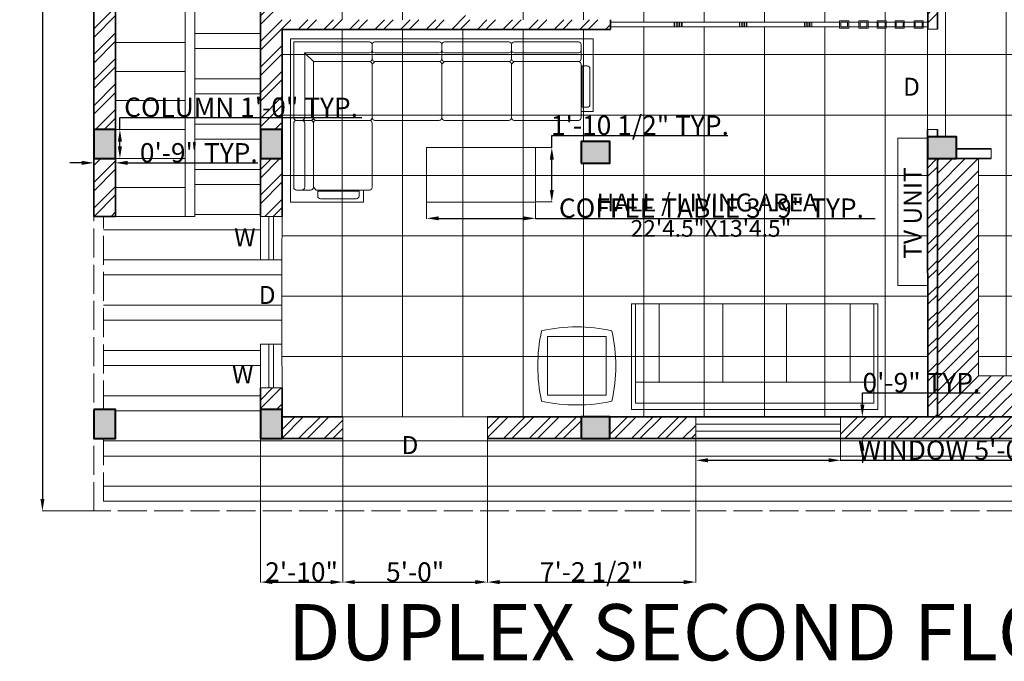
# Model space of a CAD drawing. Units: inches. Extents: x 351 to 1738, y -265 to 286.
# Tile 1 of 38: x 351 to 759, y -265 to 0. Entities that reach past the tile are written whole.
import ezdxf

# ---------------------------------------------------------------- set-up
doc = ezdxf.new("R2010")
doc.units = ezdxf.units.IN
doc.header["$MEASUREMENT"] = 0
doc.linetypes.add('ACAD_ISO02W100', pattern=[15, 12, -3])
doc.linetypes.add('ACAD_ISO03W100', pattern=[30, 12, -18])
for name, color, linetype, lineweight in [('A-ANNO-DIMS', 2, 'Continuous', 18), ('A-ANNO-SYMB', 7, 'Continuous', 18), ('A-ANNO-TEXT', 7, 'Continuous', 18), ('A-ANNO-TITL', 7, 'Continuous', 35), ('A-AREA-IDEN', 7, 'Continuous', 18), ('A-COLS', 7, 'Continuous', 40), ('A-COLS-PATT', 6, 'Continuous', 13), ('A-DOOR', 3, 'Continuous', 18), ('A-DOOR-HIDN', 3, 'ACAD_ISO03W100', 13), ('A-DOOR-OVHD', 3, 'ACAD_ISO02W100', 13), ('A-FLOR-CASE', 9, 'Continuous', 18), ('A-FLOR-CASE-PATT', 9, 'Continuous', 9), ('A-FLOR-OVHD', 1, 'ACAD_ISO02W100', 18), ('A-FLOR-PATT', 9, 'Continuous', 9), ('A-FLOR-STRS', 7, 'Continuous', 18), ('A-FURN', 18, 'Continuous', 13), ('A-GLAZ', 4, 'Continuous', 18), ('A-WALL', 7, 'Continuous', 35), ('A-WALL-PATT', 152, 'Continuous', 13), ('A-WALL-SCRN', 7, 'Continuous', 18), ('A-WALL-SCRN-PATT', 30, 'Continuous', 13)]:
    doc.layers.add(name, color=color, linetype=linetype, lineweight=lineweight)
doc.styles.add('Annotative', font='arial.ttf')
doc.styles.get("Standard").update_dxf_attribs({"font": 'arial.ttf'})
doc.dimstyles.get("Standard").update_dxf_attribs({"dimtxt": 8, "dimasz": 5, "dimexe": 0.18, "dimexo": 0.0625, "dimgap": 0.09, "dimtad": 1, "dimtoh": 1, "dimzin": 0, "dimdsep": 46, "dimlunit": 4, "dimtxsty": 'Standard', "dimcen": 0, "dimclre": 256, "dimadec": 0, "dimazin": 0, "dimtfac": 1, "dimtofl": 0, "dimtmove": 0, "dimatfit": 3, "dimfxl": 1, "dimtolj": 1, "dimtzin": 0, "dimlwe": -1, "dimarcsym": 0})

# ---------------------------------------------------------------- blocks, each defined once
blk = doc.blocks.new('*D3')
at = {"layer": 'A-ANNO-DIMS', "color": 0, "transparency": 16777216}
for p, q in [((382.09, 255.96), (360.67, 255.96)), ((382.09, -203.04), (360.67, -203.04))]:
    blk.add_line(p, q, dxfattribs=at)
at = {"layer": 'A-ANNO-DIMS', "color": 0, "lineweight": -2, "transparency": 16777216}
blk.add_line((360.85, 250.96), (360.85, -198.04), dxfattribs=at)
at = {"layer": 'A-ANNO-DIMS', "color": 0, "transparency": 16777216}
for points in [[(360.02, 250.96), (361.69, 250.96), (360.85, 255.96)], [(360.02, -198.04), (361.69, -198.04), (360.85, -203.04)]]:
    blk.add_solid(points, dxfattribs=at)
at = {"layer": 'Defpoints', "color": 0, "transparency": 16777216}
for p in [(382.16, 255.96), (360.85, -203.04), (382.16, -203.04)]:
    blk.add_point(p, dxfattribs=at)
at = {"layer": 'A-ANNO-DIMS', "color": 0, "transparency": 16777216, "insert": (356.68, 26.46), "char_height": 8, "attachment_point": 5, "rotation": 90}
blk.add_mtext('\\A1;38\'-3"', dxfattribs=at)
blk = doc.blocks.new('TABLE-COFFEE-RECT')
blk.add_lwpolyline([(0, 0), (0, 22.55), (45.11, 22.55), (45.11, 0)], close=True)
blk = doc.blocks.new('CONSOLE-TV')
blk.add_lwpolyline([(0, 0), (61, 0), (61, 12.29), (0, 12.29)], close=True)
blk = doc.blocks.new('COL-9x12')
blk.add_lwpolyline([(0, 12), (0, 0), (9, 0), (9, 12)], close=True)
blk = doc.blocks.new('WIN-60')
for p, q in [((0, 6), (60, 6)), ((0, 3), (60, 3))]:
    blk.add_line(p, q)
blk.add_lwpolyline([(60, 0), (60, 9), (0, 9), (0, 0)], close=True)
blk = doc.blocks.new('*D30')
at = {"layer": 'A-ANNO-DIMS', "color": 0, "lineweight": -2, "transparency": 16777216}
for p, q in [((392.96, -45.04), (392.96, -40.04)), ((392.96, -40.04), (493.25, -40.04)), ((392.96, -52.04), (392.96, -50.04))]:
    blk.add_line(p, q, dxfattribs=at)
at = {"layer": 'A-ANNO-DIMS', "transparency": 16777216}
for p, q in [((391.22, -45.04), (393.14, -45.04)), ((391.22, -57.04), (393.14, -57.04))]:
    blk.add_line(p, q, dxfattribs=at)
at = {"layer": 'A-ANNO-DIMS', "color": 0, "transparency": 16777216}
for points in [[(392.12, -50.04), (393.79, -50.04), (392.96, -45.04)], [(392.12, -52.04), (393.79, -52.04), (392.96, -57.04)]]:
    blk.add_solid(points, dxfattribs=at)
at = {"layer": 'Defpoints', "color": 0, "transparency": 16777216}
for p in [(391.16, -45.04), (392.96, -45.04), (391.16, -57.04)]:
    blk.add_point(p, dxfattribs=at)
at = {"layer": 'A-ANNO-DIMS', "color": 0, "transparency": 16777216, "insert": (443.15, -35.81), "char_height": 8, "attachment_point": 5}
blk.add_mtext('\\A1;COLUMN 1\'-0" TYP.', dxfattribs=at)
blk = doc.blocks.new('*D31')
at = {"layer": 'A-ANNO-DIMS', "transparency": 16777216}
for p, q in [((382.16, -57.1), (382.16, -59.02)), ((391.16, -57.1), (391.16, -59.02))]:
    blk.add_line(p, q, dxfattribs=at)
at = {"layer": 'A-ANNO-DIMS', "color": 0, "lineweight": -2, "transparency": 16777216}
for p, q in [((377.16, -58.84), (372.16, -58.84)), ((396.16, -58.84), (450.1, -58.84))]:
    blk.add_line(p, q, dxfattribs=at)
at = {"layer": 'A-ANNO-DIMS', "color": 0, "transparency": 16777216}
for points in [[(377.16, -58), (377.16, -59.67), (382.16, -58.84)], [(396.16, -58), (396.16, -59.67), (391.16, -58.84)]]:
    blk.add_solid(points, dxfattribs=at)
at = {"layer": 'Defpoints', "color": 0, "transparency": 16777216}
for p in [(382.16, -57.04), (391.16, -57.04), (391.16, -58.84)]:
    blk.add_point(p, dxfattribs=at)
at = {"layer": 'A-ANNO-DIMS', "color": 0, "transparency": 16777216, "insert": (425.63, -54.66), "char_height": 8, "attachment_point": 5}
blk.add_mtext('\\A1;0\'-9" TYP.', dxfattribs=at)
blk = doc.blocks.new('*D34')
at = {"layer": 'A-ANNO-DIMS', "transparency": 16777216}
for p, q in [((631.58, -173.1), (631.58, -182.22)), ((691.58, -173.1), (691.58, -182.22))]:
    blk.add_line(p, q, dxfattribs=at)
at = {"layer": 'A-ANNO-DIMS', "color": 0, "lineweight": -2, "transparency": 16777216}
for p, q in [((636.58, -182.04), (686.58, -182.04)), ((691.58, -182.04), (797.99, -182.04))]:
    blk.add_line(p, q, dxfattribs=at)
at = {"layer": 'A-ANNO-DIMS', "color": 0, "transparency": 16777216}
for points in [[(636.58, -181.2), (636.58, -182.87), (631.58, -182.04)], [(686.58, -181.2), (686.58, -182.87), (691.58, -182.04)]]:
    blk.add_solid(points, dxfattribs=at)
at = {"layer": 'Defpoints', "color": 0, "transparency": 16777216}
for p in [(631.58, -173.04), (691.58, -173.04), (691.58, -182.04)]:
    blk.add_point(p, dxfattribs=at)
at = {"layer": 'A-ANNO-DIMS', "color": 0, "transparency": 16777216, "insert": (747.29, -177.81), "char_height": 8, "attachment_point": 5}
blk.add_mtext('\\A1;WINDOW 5\'-0" TYP.', dxfattribs=at)
blk = doc.blocks.new('*D35')
at = {"layer": 'A-ANNO-DIMS', "color": 0, "lineweight": -2, "transparency": 16777216}
for p, q in [((700.58, -159.04), (700.58, -154.04)), ((700.58, -154.04), (749.43, -154.04)), ((700.58, -178.04), (700.58, -183.04))]:
    blk.add_line(p, q, dxfattribs=at)
at = {"layer": 'A-ANNO-DIMS', "transparency": 16777216}
for p, q in [((691.64, -164.04), (700.76, -164.04)), ((691.64, -173.04), (700.76, -173.04))]:
    blk.add_line(p, q, dxfattribs=at)
at = {"layer": 'A-ANNO-DIMS', "color": 0, "transparency": 16777216}
for points in [[(699.75, -159.04), (701.41, -159.04), (700.58, -164.04)], [(699.75, -178.04), (701.41, -178.04), (700.58, -173.04)]]:
    blk.add_solid(points, dxfattribs=at)
at = {"layer": 'Defpoints', "color": 0, "transparency": 16777216}
for p in [(691.58, -164.04), (700.58, -164.04), (691.58, -173.04)]:
    blk.add_point(p, dxfattribs=at)
at = {"layer": 'A-ANNO-DIMS', "color": 0, "transparency": 16777216, "insert": (725.05, -149.86), "char_height": 8, "attachment_point": 5}
blk.add_mtext('\\A1;0\'-9" TYP.', dxfattribs=at)
blk = doc.blocks.new('*D50')
at = {"layer": 'A-ANNO-DIMS', "transparency": 16777216}
for p, q in [((520.02, -75.12), (520.02, -82)), ((565.13, -75.12), (565.13, -82))]:
    blk.add_line(p, q, dxfattribs=at)
at = {"layer": 'A-ANNO-DIMS', "color": 0, "lineweight": -2, "transparency": 16777216}
for p, q in [((525.02, -81.82), (560.13, -81.82)), ((565.13, -81.82), (705.92, -81.82))]:
    blk.add_line(p, q, dxfattribs=at)
at = {"layer": 'A-ANNO-DIMS', "color": 0, "transparency": 16777216}
for points in [[(525.02, -80.99), (525.02, -82.65), (520.02, -81.82)], [(560.13, -80.99), (560.13, -82.65), (565.13, -81.82)]]:
    blk.add_solid(points, dxfattribs=at)
at = {"layer": 'Defpoints', "color": 0, "transparency": 16777216}
for p in [(520.02, -75.05), (565.13, -75.05), (565.13, -81.82)]:
    blk.add_point(p, dxfattribs=at)
at = {"layer": 'A-ANNO-DIMS', "color": 0, "transparency": 16777216, "insert": (638.03, -77.59), "char_height": 8, "attachment_point": 5}
blk.add_mtext('\\A1;COFFEE TABLE 3\'-9" TYP.', dxfattribs=at)
blk = doc.blocks.new('*D51')
at = {"layer": 'A-ANNO-DIMS', "color": 0, "lineweight": -2, "transparency": 16777216}
for p, q in [((571.9, -52.5), (571.9, -47.5)), ((571.9, -47.5), (644.85, -47.5)), ((571.9, -70.05), (571.9, -57.5))]:
    blk.add_line(p, q, dxfattribs=at)
at = {"layer": 'A-ANNO-DIMS', "transparency": 16777216}
for p, q in [((565.19, -52.5), (572.08, -52.5)), ((565.19, -75.05), (572.08, -75.05))]:
    blk.add_line(p, q, dxfattribs=at)
at = {"layer": 'A-ANNO-DIMS', "color": 0, "transparency": 16777216}
for points in [[(571.06, -57.5), (572.73, -57.5), (571.9, -52.5)], [(571.06, -70.05), (572.73, -70.05), (571.9, -75.05)]]:
    blk.add_solid(points, dxfattribs=at)
at = {"layer": 'Defpoints', "color": 0, "transparency": 16777216}
for p in [(565.13, -52.5), (571.9, -52.5), (565.13, -75.05)]:
    blk.add_point(p, dxfattribs=at)
at = {"layer": 'A-ANNO-DIMS', "color": 0, "transparency": 16777216, "insert": (608.42, -43.28), "char_height": 8, "attachment_point": 5}
blk.add_mtext('\\A1;1\'-10 1/2" TYP.', dxfattribs=at)
blk = doc.blocks.new('*D56')
at = {"layer": 'A-ANNO-DIMS', "transparency": 16777216}
for p, q in [((451.16, -173.1), (451.16, -232.67)), ((485.28, -173.1), (485.28, -232.67))]:
    blk.add_line(p, q, dxfattribs=at)
at = {"layer": 'A-ANNO-DIMS', "color": 0, "lineweight": -2, "transparency": 16777216}
blk.add_line((456.16, -232.49), (480.28, -232.49), dxfattribs=at)
at = {"layer": 'A-ANNO-DIMS', "color": 0, "transparency": 16777216}
for points in [[(456.16, -231.65), (456.16, -233.32), (451.16, -232.49)], [(480.28, -231.65), (480.28, -233.32), (485.28, -232.49)]]:
    blk.add_solid(points, dxfattribs=at)
at = {"layer": 'Defpoints', "color": 0, "transparency": 16777216}
for p in [(451.16, -173.04), (485.28, -173.04), (485.28, -232.49)]:
    blk.add_point(p, dxfattribs=at)
at = {"layer": 'A-ANNO-DIMS', "color": 0, "transparency": 16777216, "insert": (468.22, -228.31), "char_height": 8, "attachment_point": 5}
blk.add_mtext('\\A1;2\'-10"', dxfattribs=at)
blk = doc.blocks.new('*D57')
at = {"layer": 'A-ANNO-DIMS', "transparency": 16777216}
for p, q in [((485.28, -173.1), (485.28, -232.67)), ((545.28, -173.1), (545.28, -232.67))]:
    blk.add_line(p, q, dxfattribs=at)
at = {"layer": 'A-ANNO-DIMS', "color": 0, "lineweight": -2, "transparency": 16777216}
blk.add_line((490.28, -232.49), (540.28, -232.49), dxfattribs=at)
at = {"layer": 'A-ANNO-DIMS', "color": 0, "transparency": 16777216}
for points in [[(490.28, -231.65), (490.28, -233.32), (485.28, -232.49)], [(540.28, -231.65), (540.28, -233.32), (545.28, -232.49)]]:
    blk.add_solid(points, dxfattribs=at)
at = {"layer": 'Defpoints', "color": 0, "transparency": 16777216}
for p in [(485.28, -173.04), (545.28, -173.04), (545.28, -232.49)]:
    blk.add_point(p, dxfattribs=at)
at = {"layer": 'A-ANNO-DIMS', "color": 0, "transparency": 16777216, "insert": (515.28, -228.31), "char_height": 8, "attachment_point": 5}
blk.add_mtext('\\A1;5\'-0"', dxfattribs=at)
blk = doc.blocks.new('*D58')
at = {"layer": 'A-ANNO-DIMS', "transparency": 16777216}
for p, q in [((545.28, -173.1), (545.28, -232.67)), ((631.58, -173.1), (631.58, -232.67))]:
    blk.add_line(p, q, dxfattribs=at)
at = {"layer": 'A-ANNO-DIMS', "color": 0, "lineweight": -2, "transparency": 16777216}
blk.add_line((550.28, -232.49), (626.58, -232.49), dxfattribs=at)
at = {"layer": 'A-ANNO-DIMS', "color": 0, "transparency": 16777216}
for points in [[(550.28, -231.65), (550.28, -233.32), (545.28, -232.49)], [(626.58, -231.65), (626.58, -233.32), (631.58, -232.49)]]:
    blk.add_solid(points, dxfattribs=at)
at = {"layer": 'Defpoints', "color": 0, "transparency": 16777216}
for p in [(545.28, -173.04), (631.58, -173.04), (631.58, -232.49)]:
    blk.add_point(p, dxfattribs=at)
at = {"layer": 'A-ANNO-DIMS', "color": 0, "transparency": 16777216, "insert": (588.43, -228.26), "char_height": 8, "attachment_point": 5}
blk.add_mtext('\\A1;7\'-2 1/2"', dxfattribs=at)

msp = doc.modelspace()

# ---------------------------------------------------------------- hatches: boundary and pattern name
at = {"layer": 'A-COLS-PATT'}
h = msp.add_hatch(color=256, dxfattribs=at)
h.dxf.hatch_style = 1
h.paths.add_polyline_path([(460.155, 237.963), (451.155, 237.963), (451.155, 228.963), (460.155, 228.963)])
h.paths.add_polyline_path([(463.155, 237.963), (460.155, 237.963), (460.155, 228.963), (463.155, 228.963)])
h.paths.add_polyline_path([(391.155, 255.963), (382.155, 255.963), (382.155, 243.963), (391.155, 243.963)])
h.paths.add_polyline_path([(391.155, 210.963), (382.155, 210.963), (382.155, 198.963), (391.155, 198.963)])
h.paths.add_polyline_path([(391.155, -45.037), (382.155, -45.037), (382.155, -57.037), (391.155, -57.037)])
h.paths.add_polyline_path([(460.155, -45.037), (451.155, -45.037), (451.155, -57.037), (460.155, -57.037)])
h.paths.add_polyline_path([(460.155, -161.037), (451.155, -161.037), (451.155, -164.037), (451.155, -173.037), (460.155, -173.037)])
h.paths.add_polyline_path([(391.155, -161.037), (382.155, -161.037), (382.155, -173.037), (391.155, -173.037)])
h.paths.add_polyline_path([(596, -164.037), (584, -164.037), (584, -173.037), (596, -173.037)])
h.paths.add_polyline_path([(596, -50), (584, -50), (584, -59), (596, -59)])
h.paths.add_polyline_path([(596.155, 73.463), (592.155, 73.463), (592.155, 64.463), (596.155, 64.463)])
h.paths.add_polyline_path([(592.155, 73.463), (584.155, 73.463), (584.155, 64.463), (592.155, 64.463)])
h.paths.add_polyline_path([(596.155, 237.963), (584.155, 237.963), (584.155, 228.963), (596.155, 228.963)])
h.paths.add_polyline_path([(739.655, 237.963), (727.655, 237.963), (727.655, 228.963), (739.655, 228.963)])
h.paths.add_polyline_path([(883.515, 237.963), (871.515, 237.963), (871.515, 228.963), (883.515, 228.963)])
h.paths.add_polyline_path([(883.515, 73.463), (871.515, 73.463), (871.515, 64.463), (883.515, 64.463)])
h.paths.add_polyline_path([(731.655, 73.463), (727.655, 73.463), (727.655, 64.463), (731.655, 64.463)])
h.paths.add_polyline_path([(739.515, 73.463), (731.655, 73.463), (731.655, 64.463), (739.515, 64.463)])
h.paths.add_polyline_path([(883.515, -53.037), (871.515, -53.037), (871.515, -57.037), (883.515, -57.037)])
h.paths.add_polyline_path([(883.515, -48.037), (871.515, -48.037), (871.515, -53.037), (883.515, -53.037)])
h.paths.add_polyline_path([(739.515, -48.037), (727.515, -48.037), (727.515, -56.5), (727.516, -57.037), (739.515, -57.037)])
h.paths.add_polyline_path([(883.515, -164.037), (871.515, -164.037), (871.515, -173.037), (883.515, -173.037)])
at = {"layer": 'A-FLOR-CASE-PATT'}
h = msp.add_hatch(dxfattribs=at)
h.set_pattern_fill('ANSI31', color=256, scale=30)
h.set_pattern_definition([(45, (731.6553, -164.0373), (-2.65165, 2.65165), [])])
h.paths.add_polyline_path([(748.655, -57.037), (731.655, -57.037), (731.655, -164.037), (815.655, -164.037), (815.655, -147.037), (748.655, -147.037)])
at = {"layer": 'A-FLOR-PATT', "transparency": 33554559}
h = msp.add_hatch(dxfattribs=at)
h.set_pattern_fill('ANSI37', color=256, scale=200, angle=45)
h.set_pattern_definition([(90, (460.077, -164.037), (-25, 0), []), (180, (460.077, -164.037), (-4e-15, -25), [])])
h.paths.add_polyline_path([(727.516, -57.037), (727.515, -57.037), (727.515, -56.5), (727.5, -45), (727.5, -3.5), (727.501, -2.537), (725.797, -2.537), (725.797, -3.037), (721.988, -3.037), (721.988, -2.537), (717.916, -2.537), (717.916, -3.037), (714.106, -3.037), (714.106, -2.537), (710.487, -2.537), (710.487, -3.037), (706.677, -3.037), (706.677, -2.537), (702.965, -2.537), (702.965, -3.037), (699.155, -3.037), (699.155, -2.537), (694.965, -2.537), (694.965, -3.037), (691.155, -3.037), (691.155, -2.537), (679.655, -2.537), (678.797, -2.537), (677.776, -2.537), (676.723, -2.537), (652.655, -2.537), (651.799, -2.537), (650.778, -2.537), (649.725, -2.537), (625.877, -2.537), (624.879, -2.537), (623.857, -2.537), (622.804, -2.537), (596.155, -2.537), (596.155, -3.537), (460.155, -3.537), (460.155, -81.037), (460.077, -99.07), (460.077, -133.967), (460.155, -152.037), (460.155, -164.037), (485.277, -164.037), (545.277, -164.037), (727.655, -164.037)])
h.paths.add_polyline_path([(584, -59), (584, -50), (596, -50), (596, -59)], flags=16)
h.paths.add_polyline_path([(905.155, 204.963), (731.655, 204.963), (731.655, 73.463), (739.515, 73.463), (739.515, 64.463), (731.655, 64.463), (731.655, -3.5), (727.655, -3.5), (727.655, -3.537), (727.5, -45), (731.655, -45), (731.655, -48.037), (739.515, -48.037), (739.515, -53.037), (754, -53.037), (754, -57.037), (748.655, -57.037), (748.655, -147.037), (815.655, -147.037), (815.655, -138.5), (819.655, -138.5), (819.655, -102.5), (815.655, -102.5), (815.655, -57.037), (790, -57.037), (790, -53.037), (871.515, -53.037), (871.515, -48.037), (883.515, -48.037), (883.515, -53.037), (905.155, -53.037)])
h.paths.add_polyline_path([(871.515, 64.463), (871.515, 73.463), (883.515, 73.463), (883.515, 64.463)], flags=16)
h.paths.add_polyline_path([(727.655, 64.463), (685.515, 64.463), (685.515, 186.963), (638.155, 186.963), (638.155, 88.463), (596.155, 88.463), (596.155, 64.463), (584.155, 64.463), (584.155, 73.463), (592.155, 73.463), (592.155, 205.963), (574, 205.963), (574, 209.963), (538, 209.963), (538, 205.963), (536.5, 205.963), (536.5, 180), (489.5, 180), (489.5, 68.655), (460.155, 68.655), (460.155, 64.463), (536.155, 64.463), (536.155, 48.463), (532.155, 48.463), (532.155, 60.463), (460.155, 60.463), (460.155, 0.463), (532.155, 0.463), (532.155, 12.463), (536.155, 12.463), (536.155, 0.463), (596.155, 0.463), (596.155, -0.537), (622.655, -0.537), (623.655, -0.537), (624.655, -0.537), (625.655, -0.537), (649.655, -0.537), (650.576, -0.537), (651.576, -0.537), (652.576, -0.537), (676.655, -0.537), (677.574, -0.537), (678.574, -0.537), (679.574, -0.537), (691.155, -0.537), (691.155, -0.037), (694.965, -0.037), (694.965, -0.537), (699.155, -0.537), (699.155, -0.037), (702.965, -0.037), (702.965, -0.537), (706.677, -0.537), (706.677, -0.037), (710.487, -0.037), (710.487, -0.537), (714.106, -0.537), (714.106, -0.037), (717.916, -0.037), (717.916, -0.537), (721.988, -0.537), (721.988, -0.037), (725.797, -0.037), (725.797, -0.537), (727.655, -0.537)])
h.paths.add_polyline_path([(485.401, 6.538), (461.783, 6.538), (461.783, 51.327), (485.401, 51.327)], flags=16)
h.paths.add_polyline_path([(483.401, 8.538), (463.783, 8.538), (463.783, 49.327), (483.401, 49.327)], flags=0)
h.paths.add_polyline_path([(476.907, 30.5), (476.907, 29.5), (476.907, 26), (475.907, 26), (475.907, 29.5), (474.449, 29.5), (474.449, 26), (473.449, 26), (470.5, 26), (470.5, 27), (473.449, 27), (473.449, 29.5), (470.5, 29.5), (470.5, 32.758), (471.5, 32.758), (471.5, 30.5), (473.407, 30.5), (473.407, 32.897), (473.407, 33.897), (476.907, 33.897), (476.907, 32.897), (474.407, 32.897), (474.407, 30.5)], flags=0)
h = msp.add_hatch(dxfattribs=at)
h.set_pattern_fill('ANSI32', color=256, scale=50, angle=135)
h.set_pattern_definition([(180, (386.155, -199.037), (-2e-15, -18.75), []), (180, (379.905, -192.787), (-2e-15, -18.75), [])])
h.paths.add_polyline_path([(451.234, -133.967), (460.077, -133.967), (460.077, -99.07), (451.234, -99.07), (451.155, -81.037), (451.155, 98.963), (423.885, 98.963), (424, -81.037), (419, -81.037), (391.155, -81.037), (386.155, -81.037), (386.155, -161.037), (391.155, -161.037), (391.155, -173.037), (386.155, -173.037), (386.155, -199.037), (910.155, -199.037), (910.155, -173.037), (545.277, -173.037), (545.277, -164.037), (485.277, -164.037), (485.277, -173.037), (451.155, -173.037), (451.155, -161.037), (451.155, -152.037)])
at = {"layer": 'A-WALL-PATT'}
h = msp.add_hatch(dxfattribs=at)
h.set_pattern_fill('ANSI32', color=256, scale=20)
h.set_pattern_definition([(45, (382.155, -173.037), (-5.3033, 5.3033), []), (45, (385.691, -173.037), (-5.3033, 5.3033), [])])
h.paths.add_polyline_path([(391.155, -57.037), (382.155, -57.037), (382.155, -81.037), (391.155, -81.037)])
h.paths.add_polyline_path([(391.155, 198.963), (382.155, 198.963), (382.155, -45.037), (391.155, -45.037)])
h.paths.add_polyline_path([(391.155, 243.963), (382.155, 243.963), (382.155, 237.963), (382.155, 210.963), (391.155, 210.963)])
h.paths.add_polyline_path([(460.155, 255.963), (391.155, 255.963), (391.155, 246.963), (451.155, 246.963), (451.155, 237.963), (460.155, 237.963), (460.155, 251.963)])
h.paths.add_polyline_path([(404.155, 207.963), (391.155, 207.963), (391.155, 198.963), (404.155, 198.963)])
h.paths.add_polyline_path([(451.155, 207.963), (440.155, 207.963), (440.155, 198.963), (451.155, 198.963)])
h.paths.add_polyline_path([(460.155, 228.963), (451.155, 228.963), (451.155, 74.963), (460.155, 74.963), (460.155, 97.5)])
h.paths.add_polyline_path([(460.155, 60.463), (532.155, 60.463), (532.155, 48.463), (536.155, 48.463), (536.155, 64.463), (460.155, 64.463), (460.155, 62.963), (451.155, 62.963), (451.155, 46.258), (460.155, 46.258)])
h.paths.add_polyline_path([(460.155, -3.537), (596.155, -3.537), (596.155, 0.463), (536.155, 0.463), (536.155, 12.463), (532.155, 12.463), (532.155, 0.463), (460.155, 0.463), (460.155, 10.258), (451.155, 10.258), (451.155, -45.037), (460.155, -45.037)])
h.paths.add_polyline_path([(460.155, -57.037), (451.155, -57.037), (451.155, -81.037), (460.155, -81.037)])
h.paths.add_polyline_path([(460.155, -152.037), (451.155, -152.037), (451.155, -161.037), (460.155, -161.037)])
h.paths.add_polyline_path([(485.277, -164.037), (460.155, -164.037), (460.155, -164.5), (460.155, -173.037), (485.277, -173.037)])
h.paths.add_polyline_path([(584, -164.037), (545.277, -164.037), (545.277, -173.037), (584, -173.037)])
h.paths.add_polyline_path([(631.58, -164.037), (596, -164.037), (596, -173.037), (631.58, -173.037)])
h.paths.add_polyline_path([(871.515, -164.037), (819.655, -164.037), (819.655, -138.5), (815.655, -138.5), (815.655, -164.037), (691.58, -164.037), (691.58, -173.037), (871.515, -173.037)])
h.paths.add_polyline_path([(731.655, -57.037), (727.516, -57.037), (727.655, -164.037), (731.655, -164.037)])
h.paths.add_polyline_path([(914.155, -138), (905.155, -138), (905.155, -164.037), (883.515, -164.037), (883.515, -173.037), (914.155, -173.037)])
h.paths.add_polyline_path([(914.155, -30.189), (905.155, -30.189), (905.155, -53.037), (883.515, -53.037), (883.515, -57.037), (905.155, -57.037), (905.155, -102), (914.155, -102)])
h.paths.add_polyline_path([(871.515, -53.037), (790, -53.037), (790, -57.037), (815.655, -57.037), (815.655, -102.5), (819.655, -102.5), (819.655, -57.037), (871.515, -57.037)])
h.paths.add_polyline_path([(914.155, 120.993), (905.155, 120.993), (905.155, 29.811), (914.155, 29.811)])
h.paths.add_polyline_path([(731.655, 64.463), (727.655, 64.463), (727.655, -3.5), (731.655, -3.5)])
h.paths.add_polyline_path([(481.5, 209.963), (460.155, 209.963), (460.155, 205.963), (481.5, 205.963)])
h.paths.add_polyline_path([(538, 209.963), (517.5, 209.963), (517.5, 205.963), (538, 205.963)])
h.paths.add_polyline_path([(592.155, 209.963), (574, 209.963), (574, 205.963), (592.155, 205.963)])
h.paths.add_polyline_path([(596.155, 228.963), (592.155, 228.963), (592.155, 73.463), (596.155, 73.463)])
h.paths.add_polyline_path([(614, 237.963), (596.155, 237.963), (596.155, 228.963), (614, 228.963)])
h.paths.add_polyline_path([(677, 237.963), (650, 237.963), (650, 228.963), (677, 228.963)])
h.paths.add_polyline_path([(727.655, 237.963), (713, 237.963), (713, 228.963), (727.655, 228.963)])
h.paths.add_polyline_path([(871.515, 237.963), (739.655, 237.963), (739.655, 228.963), (871.515, 228.963)])
h.paths.add_polyline_path([(731.655, 228.963), (727.655, 228.963), (727.655, 73.463), (731.655, 73.463)])
h.paths.add_polyline_path([(914.155, 237.963), (883.515, 237.963), (883.515, 228.963), (905.155, 228.963), (905.155, 180.993), (914.155, 180.993)])
at = {"layer": 'A-WALL-SCRN-PATT'}
h = msp.add_hatch(color=256, dxfattribs=at)
h.dxf.hatch_style = 1
h.paths.add_polyline_path([(623.655, -0.537), (622.804, -0.537), (622.804, -2.537), (623.655, -2.537)])
h.paths.add_polyline_path([(625.655, -0.537), (624.879, -0.537), (624.879, -2.537), (625.655, -2.537)])
h.paths.add_polyline_path([(624.655, -0.537), (623.857, -0.537), (623.857, -2.537), (624.655, -2.537)])
h.paths.add_polyline_path([(652.576, -0.537), (651.799, -0.537), (651.799, -2.537), (652.576, -2.537)])
h.paths.add_polyline_path([(651.576, -0.537), (650.778, -0.537), (650.778, -2.537), (651.576, -2.537)])
h.paths.add_polyline_path([(650.576, -0.537), (649.725, -0.537), (649.725, -2.537), (650.576, -2.537)])
h.paths.add_polyline_path([(677.574, -0.537), (676.723, -0.537), (676.723, -2.537), (677.574, -2.537)])
h.paths.add_polyline_path([(679.574, -0.537), (678.797, -0.537), (678.797, -2.537), (679.574, -2.537)])
h.paths.add_polyline_path([(678.574, -0.537), (677.776, -0.537), (677.776, -2.537), (678.574, -2.537)])
h.paths.add_polyline_path([(694.965, -0.037), (691.155, -0.037), (691.155, -3.037), (694.965, -3.037)])
h.paths.add_polyline_path([(694.465, -2.537), (691.655, -2.537), (691.655, -0.537), (694.465, -0.537)], flags=16)
h.paths.add_polyline_path([(702.965, -0.037), (699.155, -0.037), (699.155, -3.037), (702.965, -3.037)])
h.paths.add_polyline_path([(699.655, -0.537), (702.465, -0.537), (702.465, -2.537), (699.655, -2.537)], flags=16)
h.paths.add_polyline_path([(710.487, -0.037), (706.677, -0.037), (706.677, -3.037), (710.487, -3.037)])
h.paths.add_polyline_path([(707.177, -2.537), (707.177, -0.537), (709.987, -0.537), (709.987, -2.537)], flags=16)
h.paths.add_polyline_path([(717.916, -0.037), (714.106, -0.037), (714.106, -3.037), (717.916, -3.037)])
h.paths.add_polyline_path([(717.416, -2.537), (714.606, -2.537), (714.606, -0.537), (717.416, -0.537)], flags=16)
h.paths.add_polyline_path([(725.797, -0.037), (721.988, -0.037), (721.988, -3.037), (725.797, -3.037)])
h.paths.add_polyline_path([(725.297, -2.537), (722.488, -2.537), (722.488, -0.537), (725.297, -0.537)], flags=16)

# ---------------------------------------------------------------- linework, layer by layer
at = {"layer": 'A-DOOR'}
for p, q in [((727.5, -45), (727.5, -3.5)), ((727.655, -3.5), (731.655, -3.5)), ((731.655, -45), (727.5, -45))]:
    msp.add_line(p, q, dxfattribs=at)
for points in [[(754, -53.037), (754, -57.037)], [(451.234, -99.07), (460.077, -99.07)], [(460.077, -133.967), (451.234, -133.967)], [(485.277, -164.037), (485.277, -173.037)], [(545.277, -173.037), (545.277, -164.037)]]:
    msp.add_lwpolyline(points, dxfattribs=at)
at = {"layer": 'A-DOOR-HIDN'}
msp.add_line((485.277, -164.037), (545.277, -164.037), dxfattribs=at)
at = {"layer": 'A-DOOR-OVHD'}
msp.add_line((460.077, -99.07), (460.077, -133.967), dxfattribs=at)
at = {"layer": 'A-FLOR-CASE'}
for p, q in [((748.655, -57.037), (748.655, -147.037)), ((748.655, -147.037), (815.655, -147.037))]:
    msp.add_line(p, q, dxfattribs=at)
at = {"layer": 'A-FLOR-OVHD'}
for p, q in [((382.155, -203.037), (382.155, -81.037)), ((386.155, -161.037), (386.155, -81.037)), ((386.155, -199.037), (386.155, -173.037)), ((910.155, -199.037), (386.155, -199.037)), ((914.155, -203.037), (382.155, -203.037))]:
    msp.add_line(p, q, dxfattribs=at)
at = {"layer": 'A-FLOR-STRS'}
for p, q in [((420, -81.037), (420, 162.963)), ((423.845, 162.963), (424, -81.037)), ((391.155, -9.037), (420, -9.037)), ((391.155, -21.037), (420, -21.037)), ((391.155, -33.037), (420, -33.037)), ((391.155, -45.037), (420, -45.037)), ((391.155, -57.037), (420, -57.037)), ((391.155, -69.037), (420, -69.037)), ((391.155, -81.037), (420, -81.037)), ((424, -81.037), (419, -81.037))]:
    msp.add_line(p, q, dxfattribs=at)
at = {"layer": 'A-FURN'}
for p, q in [((527.466, -8.749), (554.079, -8.749)), ((555.206, -9.877), (555.206, -15.741)), ((582.946, -8.749), (556.334, -8.749)), ((584.074, -15.741), (584.074, -9.877)), ((466.123, -41.225), (471.986, -41.225)), ((616.334, -117.241), (616.334, -149.636)), ((642.744, -117.241), (642.744, -149.636)), ((669.153, -117.241), (669.153, -149.636)), ((695.563, -117.241), (695.563, -149.636)), ((606.6, -149.636), (705.296, -149.636))]:
    msp.add_line(p, q, dxfattribs=at)
for points in [[(584.074, -37.617), (589.035, -37.617), (589.035, -7.396), (463.642, -7.396), (463.642, -75.054), (493.863, -75.054), (493.863, -70.093)], [(606.6, -117.241), (606.6, -158.426), (705.296, -158.426), (705.296, -117.241)]]:
    msp.add_lwpolyline(points, dxfattribs=at)
for points in [[(497.471, -9.877, 0.4142136), (496.343, -8.749), (464.995, -8.749), (464.995, -40.098, 0.4142136), (466.123, -41.225, 0.4142136), (464.995, -42.353), (464.995, -68.965, 0.4142136), (466.123, -70.093), (471.986, -70.093, 0.4142136), (473.114, -68.965)], [(468.378, -70.093, 0.4142136), (469.505, -68.965), (469.505, -42.353, 0.4142136), (468.378, -41.225, 0.4142136), (469.505, -40.098), (469.505, -13.485, 0.0570115), (469.476, -13.231, 0.0570115), (469.731, -13.26), (496.343, -13.26, 0.4142136), (497.471, -12.132, 0.4142136), (498.599, -13.26), (525.211, -13.26, 0.4142136), (526.339, -12.132, 0.4142136), (527.466, -13.26), (554.079, -13.26, 0.4142136), (555.206, -12.132, 0.4142136), (556.334, -13.26), (582.946, -13.26, 0.4142136), (584.074, -12.132)], [(527.466, -16.868, -0.4142136), (526.339, -15.741), (526.339, -9.877, 0.4142136), (525.211, -8.749), (498.599, -8.749, 0.4142136), (497.471, -9.877), (497.471, -15.741, 0.4142136), (498.599, -16.868)], [(473.114, -16.868), (496.343, -16.868, -0.4142136), (497.471, -17.996), (497.471, -40.098, -0.4142136), (496.343, -41.225), (474.242, -41.225, -0.4142136), (473.114, -40.098), (473.114, -16.868), (469.618, -13.373)], [(496.343, -16.868, 0.4142136), (497.471, -15.741)], [(497.471, -40.098, 0.4142136), (498.599, -41.225), (525.211, -41.225, 0.4142136), (526.339, -40.098), (526.339, -17.996, 0.4142136), (525.211, -16.868), (498.599, -16.868), (497.471, -17.996)], [(526.339, -40.098, 0.4142136), (527.466, -41.225), (554.079, -41.225, 0.4142136), (555.206, -40.098), (555.206, -17.996, 0.4142136), (554.079, -16.868), (527.466, -16.868), (526.339, -17.996)], [(555.206, -40.098, 0.4142136), (556.334, -41.225), (582.946, -41.225, 0.4142136), (584.074, -40.098), (584.074, -17.996, 0.4142136), (582.946, -16.868), (556.334, -16.868), (555.206, -17.996)], [(474.242, -41.225, 0.4142136), (473.114, -42.353), (473.114, -68.965), (474.242, -70.093), (496.343, -70.093, 0.4142136), (497.471, -68.965), (497.471, -42.353, 0.4142136), (496.343, -41.225)]]:
    msp.add_lwpolyline(points, format="xyb", dxfattribs=at)
for points in [[(584.525, -18.672), (584.525, -35.813), (586.555, -35.813, 0.4142136), (587.682, -34.685), (587.682, -19.8, 0.4142136), (586.555, -18.672)], [(474.918, -72.574, 0.4142136), (476.046, -73.701), (490.931, -73.701, 0.4142136), (492.058, -72.574), (492.058, -70.544), (474.918, -70.544)]]:
    msp.add_lwpolyline(points, format="xyb", close=True, dxfattribs=at)
msp.add_lwpolyline([(707, -117.241), (707, -161), (604.897, -161), (604.897, -117.241)], close=True, dxfattribs=at)
at = {"layer": 'A-FURN', "ltscale": 10}
msp.add_lwpolyline([(570.092, -130.808), (570.092, -155.119), (594.402, -155.119), (594.402, -130.808)], close=True, dxfattribs=at)
at = {"layer": 'A-FURN'}
for centre, start, end in [((527.466, -9.877), 90, 180), ((554.079, -9.877), 0, 90), ((556.334, -9.877), 90, 180), ((582.946, -9.877), 0, 90), ((525.211, -15.741), 270, 0), ((554.079, -15.741), 270, 0), ((556.334, -15.741), 180, 270), ((582.946, -15.741), 270, 0), ((471.986, -40.098), 270, 0), ((471.986, -42.353), 0, 90)]:
    msp.add_arc(centre, 1.128, start, end, dxfattribs=at)
at = {"layer": 'A-FURN', "ltscale": 10}
for centre, start, end in [((634.44, -142.963), 167.67866, 192.32134), ((582.247, -195.156), 77.67866, 102.32134), ((530.054, -142.963), 347.67866, 12.32134), ((582.247, -90.771), 257.67866, 282.32134)]:
    msp.add_arc(centre, 68.353, start, end, dxfattribs=at)
at = {"layer": 'A-GLAZ'}
for p, q in [((451.234, -99.07), (451.155, -81.037)), ((451.155, -81.037), (460.155, -81.037)), ((454.655, -99.07), (454.655, -81.037)), ((456.655, -99.07), (456.655, -81.037)), ((460.155, -81.037), (460.077, -99.07)), ((451.155, -152.037), (451.234, -133.967)), ((451.234, -133.967), (460.077, -133.967)), ((454.655, -152.037), (454.655, -133.967)), ((456.655, -152.037), (456.655, -133.967)), ((460.077, -133.967), (460.155, -152.037)), ((451.155, -152.037), (460.155, -152.037))]:
    msp.add_line(p, q, dxfattribs=at)
at = {"layer": 'A-WALL'}
for p, q in [((382.155, 255.963), (382.155, -81.037)), ((451.155, 246.963), (451.155, -81.037)), ((727.655, 228.963), (727.655, -3.537)), ((391.155, 198.963), (391.155, -81.037)), ((731.655, 64.463), (731.655, -3.5)), ((596.155, 0.463), (596.155, -3.537)), ((460.155, -3.537), (596.155, -3.537)), ((460.155, -3.537), (460.155, -81.037)), ((727.5, -45), (727.655, -164.037)), ((731.655, -45), (731.655, -48.037)), ((727.655, -57.037), (754, -57.037)), ((731.655, -57.037), (731.655, -164.037)), ((739.515, -53.037), (754, -53.037)), ((382.155, -81.037), (391.155, -81.037)), ((451.155, -164.037), (451.155, -152.037)), ((460.155, -152.037), (460.155, -164.5)), ((460.155, -164.037), (485.277, -164.037)), ((545.277, -164.037), (815.655, -164.037)), ((382.155, -173.037), (391.155, -173.037)), ((451.155, -173.037), (485.277, -173.037)), ((545.277, -173.037), (914.155, -173.037))]:
    msp.add_line(p, q, dxfattribs=at)
at = {"layer": 'A-WALL-SCRN'}
for p, q in [((596.155, -0.537), (622.655, -0.537)), ((596.155, -2.537), (622.655, -2.537)), ((622.655, -2.537), (622.655, -0.537)), ((625.877, -0.537), (625.877, -2.537)), ((625.877, -0.537), (649.655, -0.537)), ((625.877, -2.537), (649.655, -2.537)), ((649.655, -2.537), (649.655, -0.537)), ((652.655, -2.537), (652.655, -0.537)), ((652.655, -0.537), (676.655, -0.537)), ((652.655, -2.537), (676.655, -2.537)), ((676.655, -2.537), (676.655, -0.537)), ((679.655, -2.537), (679.655, -0.537)), ((679.655, -0.537), (691.155, -0.537)), ((679.655, -2.537), (691.155, -2.537)), ((694.965, -0.537), (699.155, -0.537)), ((694.965, -2.537), (699.155, -2.537)), ((699.655, -0.537), (702.465, -0.537)), ((699.655, -2.537), (702.465, -2.537)), ((702.965, -0.537), (706.677, -0.537)), ((702.965, -2.537), (706.677, -2.537)), ((707.177, -0.537), (709.987, -0.537)), ((707.177, -2.537), (709.987, -2.537)), ((710.487, -0.537), (714.106, -0.537)), ((710.487, -2.537), (714.106, -2.537)), ((714.606, -0.537), (717.416, -0.537)), ((714.606, -2.537), (717.416, -2.537)), ((717.916, -0.537), (721.988, -0.537)), ((717.916, -2.537), (721.988, -2.537)), ((722.488, -0.537), (725.297, -0.537)), ((722.488, -2.537), (725.297, -2.537)), ((725.797, -0.537), (727.655, -0.537)), ((725.797, -2.537), (727.655, -2.537))]:
    msp.add_line(p, q, dxfattribs=at)
for points in [[(622.804, -0.537), (622.804, -2.537), (623.655, -2.537), (623.655, -0.537)], [(623.857, -0.537), (623.857, -2.537), (624.655, -2.537), (624.655, -0.537)], [(624.879, -0.537), (624.879, -2.537), (625.655, -2.537), (625.655, -0.537)], [(649.725, -0.537), (649.725, -2.537), (650.576, -2.537), (650.576, -0.537)], [(650.778, -0.537), (650.778, -2.537), (651.576, -2.537), (651.576, -0.537)], [(651.799, -0.537), (651.799, -2.537), (652.576, -2.537), (652.576, -0.537)], [(676.723, -0.537), (676.723, -2.537), (677.574, -2.537), (677.574, -0.537)], [(677.776, -0.537), (677.776, -2.537), (678.574, -2.537), (678.574, -0.537)], [(678.797, -0.537), (678.797, -2.537), (679.574, -2.537), (679.574, -0.537)], [(691.155, -3.037), (694.965, -3.037), (694.965, -0.037), (691.155, -0.037)], [(691.655, -2.537), (694.465, -2.537), (694.465, -0.537), (691.655, -0.537)], [(699.155, -3.037), (702.965, -3.037), (702.965, -0.037), (699.155, -0.037)], [(699.655, -2.537), (702.465, -2.537), (702.465, -0.537), (699.655, -0.537)], [(706.677, -3.037), (710.487, -3.037), (710.487, -0.037), (706.677, -0.037)], [(714.106, -3.037), (717.916, -3.037), (717.916, -0.037), (714.106, -0.037)], [(721.988, -3.037), (725.797, -3.037), (725.797, -0.037), (721.988, -0.037)]]:
    msp.add_lwpolyline(points, close=True, dxfattribs=at)
for points in [[(707.177, -0.537), (707.177, -2.537)], [(709.987, -2.537), (709.987, -0.537)], [(714.606, -0.537), (714.606, -2.537)], [(717.416, -2.537), (717.416, -0.537)], [(722.488, -0.537), (722.488, -2.537)], [(725.297, -2.537), (725.297, -0.537)]]:
    msp.add_lwpolyline(points, dxfattribs=at)

# ---------------------------------------------------------------- block references
at = {"layer": 'A-COLS'}
for p in [(382.155, -57.037), (451.155, -57.037), (382.155, -173.037), (451.155, -173.037)]:
    msp.add_blockref('COL-9x12', p, dxfattribs=at)
for p, rotation in [((739.515, -57.038), 90.00000000000006), ((596, -59), 90.00000000000047), ((596, -173.038), 90.00000000000047)]:
    msp.add_blockref('COL-9x12', p, dxfattribs=dict(at, rotation=rotation))
at = {"layer": 'A-FLOR-CASE', "rotation": 89.99999999999996}
msp.add_blockref('CONSOLE-TV', (727.584, -109.627), dxfattribs=at)
at = {"layer": 'A-FURN'}
msp.add_blockref('TABLE-COFFEE-RECT', (520.024, -75.054), dxfattribs=at)
at = {"layer": 'A-GLAZ'}
msp.add_blockref('WIN-60', (631.58, -173.037), dxfattribs=at)

# ---------------------------------------------------------------- texts
at = {"layer": 'A-ANNO-SYMB', "style": 'Annotative'}
for s, p in [('D', (717.457, -31.024)), ('W', (440.265, -93.38)), ('D', (450.474, -117.283)), ('W', (439.381, -150.135)), ('D', (509.627, -179.448))]:
    msp.add_text(s, height=7.433, dxfattribs=at).set_placement(p)
at = {"layer": 'A-ANNO-TEXT', "style": 'Annotative'}
msp.add_text('TV UNIT', height=7.4326, rotation=90, dxfattribs=at).set_placement((725.162, -98.551))
at = {"layer": 'A-ANNO-TITL', "style": 'Annotative'}
msp.add_text('DUPLEX SECOND FLOOR', height=23.27476, dxfattribs=at).set_placement((462.522, -264.89))
at = {"layer": 'A-AREA-IDEN', "style": 'Annotative'}
for s, height, p in [('HALL / LIVING AREA', 7.43256, (590.404, -78.98)), ('22\'4.5"X13\'4.5"', 6.90137, (604.557, -89.437))]:
    msp.add_text(s, height=height, dxfattribs=at).set_placement(p)

# ---------------------------------------------------------------- dimensions: what is measured, and where the dimension line sits
at = {"layer": 'A-ANNO-DIMS'}
dim = msp.add_linear_dim(base=(360.852, -203.037), p1=(382.155, 255.963), p2=(382.155, -203.037), angle=90, dimstyle='Standard', override={"dimclrd": 0, "dimclre": 0, "dimclrt": 0}, dxfattribs=at)
dim.commit()
dim.dimension.update_dxf_attribs({"geometry": '*D3', "text_midpoint": (360.852, 26.463), "dimtype": 160})
for base, p1, p2, text, picture, middle in [((392.955, -45.037), (391.155, -57.037), (391.155, -45.037), 'COLUMN <> TYP.', '*D30', (443.149, -35.808)), ((571.895, -52.502), (565.129, -75.054), (565.129, -52.502), '<> TYP.', '*D51', (608.419, -43.275)), ((700.58, -164.037), (691.58, -173.037), (691.58, -164.037), '<> TYP.', '*D35', (725.052, -149.863))]:
    dim = msp.add_linear_dim(base=base, p1=p1, p2=p2, angle=90, text=text, dimstyle='Standard', override={"dimdec": 1, "dimlfac": 1, "dimrnd": 0, "dimzin": 1, "dimdsep": 46, "dimlunit": 4, "dimfrac": 2}, dxfattribs=at)
    dim.commit()
    dim.dimension.update_dxf_attribs({"geometry": picture, "text_midpoint": middle})
for base, p1, p2, text, picture, middle in [((391.155, -58.837), (382.155, -57.037), (391.155, -57.037), '<> TYP.', '*D31', (425.627, -54.663)), ((565.129, -81.82), (520.024, -75.054), (565.129, -75.054), 'COFFEE TABLE <> TYP.', '*D50', (638.026, -77.588)), ((691.58, -182.037), (631.58, -173.037), (691.58, -173.037), 'WINDOW <> TYP.', '*D34', (747.286, -177.808))]:
    dim = msp.add_linear_dim(base=base, p1=p1, p2=p2, text=text, dimstyle='Standard', override={"dimdec": 1, "dimlfac": 1, "dimrnd": 0, "dimzin": 1, "dimdsep": 46, "dimlunit": 4, "dimfrac": 2}, dxfattribs=at)
    dim.commit()
    dim.dimension.update_dxf_attribs({"geometry": picture, "text_midpoint": middle})
for base, p1, p2, picture, middle in [((485.277, -232.487), (451.155, -173.037), (485.277, -173.037), '*D56', (468.216, -228.313)), ((545.277, -232.487), (485.277, -173.037), (545.277, -173.037), '*D57', (515.277, -228.313)), ((631.58, -232.487), (545.277, -173.037), (631.58, -173.037), '*D58', (588.428, -228.261))]:
    dim = msp.add_linear_dim(base=base, p1=p1, p2=p2, dimstyle='Standard', override={"dimdec": 1, "dimlfac": 1, "dimrnd": 0, "dimzin": 1, "dimdsep": 46, "dimlunit": 4, "dimfrac": 2}, dxfattribs=at)
    dim.commit()
    dim.dimension.update_dxf_attribs({"geometry": picture, "text_midpoint": middle})

doc.saveas('drawing.dxf')
